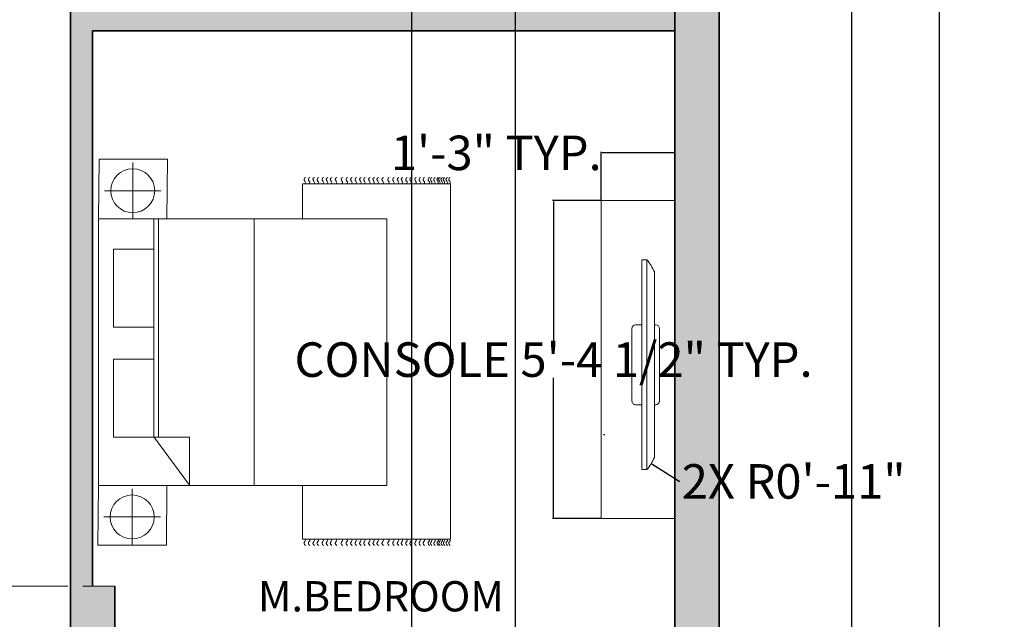
# Model space of a CAD drawing. Units: inches. Extents: x -17 to 892, y -721 to 172.
# Tile 10 of 11: x 655 to 854, y -115 to 7. Entities that reach past the tile are written whole.
import ezdxf

# ---------------------------------------------------------------- set-up
doc = ezdxf.new("R2010")
doc.units = ezdxf.units.IN
doc.header["$MEASUREMENT"] = 0
doc.linetypes.add('ACAD_ISO02W100', pattern=[15, 12, -3])
doc.layers.get('0').update_dxf_attribs({"color": 14})
for name, color, linetype, lineweight in [('A-ANNO-DIMS', 2, 'Continuous', 18), ('A-AREA-IDEN', 7, 'Continuous', 18), ('A-EQPM', 8, 'Continuous', 18), ('A-FLOR-CASE', 252, 'Continuous', 18), ('A-FLOR-OVHD', 252, 'ACAD_ISO02W100', 18), ('A-WALL-PATT', 14, 'Continuous', 13), ('furniture', 252, 'Continuous', 18), ('walls', 252, 'Continuous', 35)]:
    doc.layers.add(name, color=color, linetype=linetype, lineweight=lineweight)
doc.layers.add('A-COLS-PATT', color=254, linetype='Continuous', lineweight=13, true_color=0xd7ebd2)
doc.styles.get("Standard").update_dxf_attribs({"font": 'arial.ttf'})
doc.dimstyles.get("Standard").update_dxf_attribs({"dimtxt": 7, "dimasz": 0.18, "dimexe": 0.18, "dimexo": 0.0625, "dimgap": 0.09, "dimtad": 0, "dimtih": 1, "dimtoh": 1, "dimzin": 0, "dimdsep": 46, "dimlunit": 3, "dimtxsty": 'Standard', "dimcen": 0.09, "dimadec": 0, "dimazin": 0, "dimtfac": 1, "dimtofl": 0, "dimtmove": 0, "dimatfit": 3, "dimfxl": 1, "dimtolj": 1, "dimtzin": 0, "dimarcsym": 0})

# ---------------------------------------------------------------- blocks, each defined once
blk = doc.blocks.new('CARPET')
at = {"layer": 'furniture'}
for p, q in [((-51.53, -98.11), (-51.53, -55.12)), ((-51.53, -55.12), (-41.27, -55.12)), ((36, -55.12), (51.55, -55.12)), ((51.55, -55.12), (51.55, -98.11)), ((51.55, -98.11), (-51.53, -98.11))]:
    blk.add_line(p, q, dxfattribs=at)
for points, knots in [([(-53.37, -55.99), (-53.22, -55.8), (-52.9, -55.41), (-52.34, -55.8), (-51.89, -56.08), (-51.65, -55.91), (-51.53, -55.83)], [0, 0, 0, 0, 0.653278, 1.290138, 1.740457, 2.114451, 2.114451, 2.114451, 2.114451]), ([(-53.37, -57.26), (-53.22, -57.07), (-52.9, -56.67), (-52.34, -57.07), (-51.89, -57.35), (-51.65, -57.17), (-51.53, -57.1)], [0, 0, 0, 0, 0.653278, 1.290138, 1.740457, 2.114451, 2.114451, 2.114451, 2.114451]), ([(53.37, -55.99), (53.22, -55.8), (52.9, -55.41), (52.34, -55.8), (51.89, -56.08), (51.65, -55.91), (51.53, -55.83)], [0, 0, 0, 0, 0.653278, 1.290138, 1.740457, 2.114451, 2.114451, 2.114451, 2.114451]), ([(53.37, -57.26), (53.22, -57.07), (52.9, -56.67), (52.34, -57.07), (51.89, -57.35), (51.65, -57.17), (51.53, -57.1)], [0, 0, 0, 0, 0.653278, 1.290138, 1.740457, 2.114451, 2.114451, 2.114451, 2.114451]), ([(-53.37, -58.59), (-53.22, -58.4), (-52.9, -58.01), (-52.34, -58.4), (-51.89, -58.68), (-51.65, -58.5), (-51.53, -58.43)], [0, 0, 0, 0, 0.653278, 1.290138, 1.740457, 2.114451, 2.114451, 2.114451, 2.114451]), ([(-53.37, -59.78), (-53.22, -59.58), (-52.9, -59.19), (-52.34, -59.58), (-51.89, -59.86), (-51.65, -59.69), (-51.53, -59.61)], [0, 0, 0, 0, 0.653278, 1.290138, 1.740457, 2.114451, 2.114451, 2.114451, 2.114451]), ([(53.37, -58.59), (53.22, -58.4), (52.9, -58.01), (52.34, -58.4), (51.89, -58.68), (51.65, -58.5), (51.53, -58.43)], [0, 0, 0, 0, 0.653278, 1.290138, 1.740457, 2.114451, 2.114451, 2.114451, 2.114451]), ([(53.37, -59.78), (53.22, -59.58), (52.9, -59.19), (52.34, -59.58), (51.89, -59.86), (51.65, -59.69), (51.53, -59.61)], [0, 0, 0, 0, 0.653278, 1.290138, 1.740457, 2.114451, 2.114451, 2.114451, 2.114451]), ([(-53.37, -61.22), (-53.22, -61.02), (-52.9, -60.63), (-52.34, -61.02), (-51.89, -61.3), (-51.65, -61.13), (-51.53, -61.05)], [0, 0, 0, 0, 0.653278, 1.290138, 1.740457, 2.114451, 2.114451, 2.114451, 2.114451]), ([(-53.37, -62.44), (-53.22, -62.25), (-52.9, -61.86), (-52.34, -62.25), (-51.89, -62.53), (-51.65, -62.36), (-51.53, -62.28)], [0, 0, 0, 0, 0.653278, 1.290138, 1.740457, 2.114451, 2.114451, 2.114451, 2.114451]), ([(53.37, -61.22), (53.22, -61.02), (52.9, -60.63), (52.34, -61.02), (51.89, -61.3), (51.65, -61.13), (51.53, -61.05)], [0, 0, 0, 0, 0.653278, 1.290138, 1.740457, 2.114451, 2.114451, 2.114451, 2.114451]), ([(53.37, -62.44), (53.22, -62.25), (52.9, -61.86), (52.34, -62.25), (51.89, -62.53), (51.65, -62.36), (51.53, -62.28)], [0, 0, 0, 0, 0.653278, 1.290138, 1.740457, 2.114451, 2.114451, 2.114451, 2.114451]), ([(-53.37, -63.63), (-53.22, -63.43), (-52.9, -63.04), (-52.34, -63.43), (-51.89, -63.72), (-51.65, -63.54), (-51.53, -63.46)], [0, 0, 0, 0, 0.653278, 1.290138, 1.740457, 2.114451, 2.114451, 2.114451, 2.114451]), ([(-53.37, -65.07), (-53.22, -64.87), (-52.9, -64.48), (-52.34, -64.87), (-51.89, -65.15), (-51.65, -64.98), (-51.53, -64.9)], [0, 0, 0, 0, 0.653278, 1.290138, 1.740457, 2.114451, 2.114451, 2.114451, 2.114451]), ([(53.37, -63.63), (53.22, -63.43), (52.9, -63.04), (52.34, -63.43), (51.89, -63.72), (51.65, -63.54), (51.53, -63.46)], [0, 0, 0, 0, 0.653278, 1.290138, 1.740457, 2.114451, 2.114451, 2.114451, 2.114451]), ([(53.37, -65.07), (53.22, -64.87), (52.9, -64.48), (52.34, -64.87), (51.89, -65.15), (51.65, -64.98), (51.53, -64.9)], [0, 0, 0, 0, 0.653278, 1.290138, 1.740457, 2.114451, 2.114451, 2.114451, 2.114451]), ([(-53.37, -66.76), (-53.22, -66.56), (-52.9, -66.17), (-52.34, -66.56), (-51.89, -66.84), (-51.65, -66.67), (-51.53, -66.59)], [0, 0, 0, 0, 0.653278, 1.290138, 1.740457, 2.114451, 2.114451, 2.114451, 2.114451]), ([(-53.37, -68.2), (-53.22, -68), (-52.9, -67.61), (-52.34, -68), (-51.89, -68.28), (-51.65, -68.11), (-51.53, -68.03)], [0, 0, 0, 0, 0.653278, 1.290138, 1.740457, 2.114451, 2.114451, 2.114451, 2.114451]), ([(53.37, -66.76), (53.22, -66.56), (52.9, -66.17), (52.34, -66.56), (51.89, -66.84), (51.65, -66.67), (51.53, -66.59)], [0, 0, 0, 0, 0.653278, 1.290138, 1.740457, 2.114451, 2.114451, 2.114451, 2.114451]), ([(53.37, -68.2), (53.22, -68), (52.9, -67.61), (52.34, -68), (51.89, -68.28), (51.65, -68.11), (51.53, -68.03)], [0, 0, 0, 0, 0.653278, 1.290138, 1.740457, 2.114451, 2.114451, 2.114451, 2.114451]), ([(-53.37, -69.53), (-53.22, -69.33), (-52.9, -68.94), (-52.34, -69.33), (-51.89, -69.61), (-51.65, -69.44), (-51.53, -69.36)], [0, 0, 0, 0, 0.653278, 1.290138, 1.740457, 2.114451, 2.114451, 2.114451, 2.114451]), ([(-53.37, -70.79), (-53.22, -70.6), (-52.9, -70.21), (-52.34, -70.6), (-51.89, -70.88), (-51.65, -70.7), (-51.53, -70.63)], [0, 0, 0, 0, 0.653278, 1.290138, 1.740457, 2.114451, 2.114451, 2.114451, 2.114451]), ([(53.37, -69.53), (53.22, -69.33), (52.9, -68.94), (52.34, -69.33), (51.89, -69.61), (51.65, -69.44), (51.53, -69.36)], [0, 0, 0, 0, 0.653278, 1.290138, 1.740457, 2.114451, 2.114451, 2.114451, 2.114451]), ([(53.37, -70.79), (53.22, -70.6), (52.9, -70.21), (52.34, -70.6), (51.89, -70.88), (51.65, -70.7), (51.53, -70.63)], [0, 0, 0, 0, 0.653278, 1.290138, 1.740457, 2.114451, 2.114451, 2.114451, 2.114451]), ([(-53.37, -72.12), (-53.22, -71.93), (-52.9, -71.54), (-52.34, -71.93), (-51.89, -72.21), (-51.65, -72.04), (-51.53, -71.96)], [0, 0, 0, 0, 0.653278, 1.290138, 1.740457, 2.114451, 2.114451, 2.114451, 2.114451]), ([(-53.37, -73.31), (-53.22, -73.11), (-52.9, -72.72), (-52.34, -73.11), (-51.89, -73.4), (-51.65, -73.22), (-51.53, -73.14)], [0, 0, 0, 0, 0.653278, 1.290138, 1.740457, 2.114451, 2.114451, 2.114451, 2.114451]), ([(53.37, -72.12), (53.22, -71.93), (52.9, -71.54), (52.34, -71.93), (51.89, -72.21), (51.65, -72.04), (51.53, -71.96)], [0, 0, 0, 0, 0.653278, 1.290138, 1.740457, 2.114451, 2.114451, 2.114451, 2.114451]), ([(53.37, -73.31), (53.22, -73.11), (52.9, -72.72), (52.34, -73.11), (51.89, -73.4), (51.65, -73.22), (51.53, -73.14)], [0, 0, 0, 0, 0.653278, 1.290138, 1.740457, 2.114451, 2.114451, 2.114451, 2.114451]), ([(-53.37, -74.75), (-53.22, -74.55), (-52.9, -74.16), (-52.34, -74.55), (-51.89, -74.83), (-51.65, -74.66), (-51.53, -74.58)], [0, 0, 0, 0, 0.653278, 1.290138, 1.740457, 2.114451, 2.114451, 2.114451, 2.114451]), ([(-53.37, -75.98), (-53.22, -75.78), (-52.9, -75.39), (-52.34, -75.78), (-51.89, -76.06), (-51.65, -75.89), (-51.53, -75.81)], [0, 0, 0, 0, 0.653278, 1.290138, 1.740457, 2.114451, 2.114451, 2.114451, 2.114451]), ([(-53.37, -77.16), (-53.22, -76.96), (-52.9, -76.57), (-52.34, -76.96), (-51.89, -77.25), (-51.65, -77.07), (-51.53, -76.99)], [0, 0, 0, 0, 0.653278, 1.290138, 1.740457, 2.114451, 2.114451, 2.114451, 2.114451]), ([(53.37, -74.75), (53.22, -74.55), (52.9, -74.16), (52.34, -74.55), (51.89, -74.83), (51.65, -74.66), (51.53, -74.58)], [0, 0, 0, 0, 0.653278, 1.290138, 1.740457, 2.114451, 2.114451, 2.114451, 2.114451]), ([(53.37, -75.98), (53.22, -75.78), (52.9, -75.39), (52.34, -75.78), (51.89, -76.06), (51.65, -75.89), (51.53, -75.81)], [0, 0, 0, 0, 0.653278, 1.290138, 1.740457, 2.114451, 2.114451, 2.114451, 2.114451]), ([(53.37, -77.16), (53.22, -76.96), (52.9, -76.57), (52.34, -76.96), (51.89, -77.25), (51.65, -77.07), (51.53, -76.99)], [0, 0, 0, 0, 0.653278, 1.290138, 1.740457, 2.114451, 2.114451, 2.114451, 2.114451]), ([(-53.37, -78.6), (-53.22, -78.4), (-52.9, -78.01), (-52.34, -78.4), (-51.89, -78.68), (-51.65, -78.51), (-51.53, -78.43)], [0, 0, 0, 0, 0.653278, 1.290138, 1.740457, 2.114451, 2.114451, 2.114451, 2.114451]), ([(-53.37, -80.29), (-53.22, -80.09), (-52.9, -79.7), (-52.34, -80.09), (-51.89, -80.37), (-51.65, -80.2), (-51.53, -80.12)], [0, 0, 0, 0, 0.653278, 1.290138, 1.740457, 2.114451, 2.114451, 2.114451, 2.114451]), ([(53.37, -78.6), (53.22, -78.4), (52.9, -78.01), (52.34, -78.4), (51.89, -78.68), (51.65, -78.51), (51.53, -78.43)], [0, 0, 0, 0, 0.653278, 1.290138, 1.740457, 2.114451, 2.114451, 2.114451, 2.114451]), ([(53.37, -80.29), (53.22, -80.09), (52.9, -79.7), (52.34, -80.09), (51.89, -80.37), (51.65, -80.2), (51.53, -80.12)], [0, 0, 0, 0, 0.653278, 1.290138, 1.740457, 2.114451, 2.114451, 2.114451, 2.114451]), ([(-53.37, -81.73), (-53.22, -81.53), (-52.9, -81.14), (-52.34, -81.53), (-51.89, -81.81), (-51.65, -81.64), (-51.53, -81.56)], [0, 0, 0, 0, 0.653278, 1.290138, 1.740457, 2.114451, 2.114451, 2.114451, 2.114451]), ([(-53.37, -83.06), (-53.22, -82.86), (-52.9, -82.47), (-52.34, -82.86), (-51.89, -83.14), (-51.65, -82.97), (-51.53, -82.89)], [0, 0, 0, 0, 0.653278, 1.290138, 1.740457, 2.114451, 2.114451, 2.114451, 2.114451]), ([(53.37, -81.73), (53.22, -81.53), (52.9, -81.14), (52.34, -81.53), (51.89, -81.81), (51.65, -81.64), (51.53, -81.56)], [0, 0, 0, 0, 0.653278, 1.290138, 1.740457, 2.114451, 2.114451, 2.114451, 2.114451]), ([(53.37, -83.06), (53.22, -82.86), (52.9, -82.47), (52.34, -82.86), (51.89, -83.14), (51.65, -82.97), (51.53, -82.89)], [0, 0, 0, 0, 0.653278, 1.290138, 1.740457, 2.114451, 2.114451, 2.114451, 2.114451]), ([(-53.37, -84.18), (-53.22, -83.99), (-52.9, -83.6), (-52.34, -83.99), (-51.89, -84.27), (-51.65, -84.09), (-51.53, -84.02)], [0, 0, 0, 0, 0.653278, 1.290138, 1.740457, 2.114451, 2.114451, 2.114451, 2.114451]), ([(-53.37, -85.51), (-53.22, -85.32), (-52.9, -84.93), (-52.34, -85.32), (-51.89, -85.6), (-51.65, -85.42), (-51.53, -85.35)], [0, 0, 0, 0, 0.653278, 1.290138, 1.740457, 2.114451, 2.114451, 2.114451, 2.114451]), ([(53.37, -84.18), (53.22, -83.99), (52.9, -83.6), (52.34, -83.99), (51.89, -84.27), (51.65, -84.09), (51.53, -84.02)], [0, 0, 0, 0, 0.653278, 1.290138, 1.740457, 2.114451, 2.114451, 2.114451, 2.114451]), ([(53.37, -85.51), (53.22, -85.32), (52.9, -84.93), (52.34, -85.32), (51.89, -85.6), (51.65, -85.42), (51.53, -85.35)], [0, 0, 0, 0, 0.653278, 1.290138, 1.740457, 2.114451, 2.114451, 2.114451, 2.114451]), ([(-53.37, -86.7), (-53.22, -86.5), (-52.9, -86.11), (-52.34, -86.5), (-51.89, -86.78), (-51.65, -86.61), (-51.53, -86.53)], [0, 0, 0, 0, 0.653278, 1.290138, 1.740457, 2.114451, 2.114451, 2.114451, 2.114451]), ([(-53.37, -88.14), (-53.22, -87.94), (-52.9, -87.55), (-52.34, -87.94), (-51.89, -88.22), (-51.65, -88.05), (-51.53, -87.97)], [0, 0, 0, 0, 0.653278, 1.290138, 1.740457, 2.114451, 2.114451, 2.114451, 2.114451]), ([(53.37, -86.7), (53.22, -86.5), (52.9, -86.11), (52.34, -86.5), (51.89, -86.78), (51.65, -86.61), (51.53, -86.53)], [0, 0, 0, 0, 0.653278, 1.290138, 1.740457, 2.114451, 2.114451, 2.114451, 2.114451]), ([(53.37, -88.14), (53.22, -87.94), (52.9, -87.55), (52.34, -87.94), (51.89, -88.22), (51.65, -88.05), (51.53, -87.97)], [0, 0, 0, 0, 0.653278, 1.290138, 1.740457, 2.114451, 2.114451, 2.114451, 2.114451]), ([(-53.37, -89.36), (-53.22, -89.17), (-52.9, -88.78), (-52.34, -89.17), (-51.89, -89.45), (-51.65, -89.28), (-51.53, -89.2)], [0, 0, 0, 0, 0.653278, 1.290138, 1.740457, 2.114451, 2.114451, 2.114451, 2.114451]), ([(-53.37, -90.55), (-53.22, -90.35), (-52.9, -89.96), (-52.34, -90.35), (-51.89, -90.64), (-51.65, -90.46), (-51.53, -90.38)], [0, 0, 0, 0, 0.653278, 1.290138, 1.740457, 2.114451, 2.114451, 2.114451, 2.114451]), ([(53.37, -89.36), (53.22, -89.17), (52.9, -88.78), (52.34, -89.17), (51.89, -89.45), (51.65, -89.28), (51.53, -89.2)], [0, 0, 0, 0, 0.653278, 1.290138, 1.740457, 2.114451, 2.114451, 2.114451, 2.114451]), ([(53.37, -90.55), (53.22, -90.35), (52.9, -89.96), (52.34, -90.35), (51.9, -90.63), (51.66, -90.47), (51.55, -90.4)], [0, 0, 0, 0, 0.653278, 1.290138, 1.740457, 2.0926, 2.0926, 2.0926, 2.0926]), ([(-53.37, -91.99), (-53.22, -91.79), (-52.9, -91.4), (-52.34, -91.79), (-51.89, -92.07), (-51.65, -91.9), (-51.53, -91.82)], [0, 0, 0, 0, 0.653278, 1.290138, 1.740457, 2.114451, 2.114451, 2.114451, 2.114451]), ([(-53.37, -92.69), (-53.22, -92.48), (-52.9, -92.08), (-52.35, -92.49), (-51.89, -92.77), (-51.65, -92.6), (-51.53, -92.52)], [0, 0, 0, 0, 0.663904, 1.307406, 1.757725, 2.131719, 2.131719, 2.131719, 2.131719]), ([(-53.37, -93.61), (-53.22, -93.42), (-52.9, -93.03), (-52.34, -93.42), (-51.89, -93.7), (-51.65, -93.52), (-51.53, -93.45)], [0, 0, 0, 0, 0.653278, 1.290138, 1.740457, 2.114451, 2.114451, 2.114451, 2.114451]), ([(-53.37, -94.55), (-53.22, -94.35), (-52.9, -93.96), (-52.34, -94.35), (-51.89, -94.63), (-51.65, -94.46), (-51.53, -94.38)], [0, 0, 0, 0, 0.653278, 1.290138, 1.740457, 2.114451, 2.114451, 2.114451, 2.114451]), ([(53.37, -91.99), (53.22, -91.79), (52.9, -91.4), (52.34, -91.79), (51.9, -92.07), (51.66, -91.91), (51.55, -91.83)], [0, 0, 0, 0, 0.653278, 1.290138, 1.740457, 2.0926, 2.0926, 2.0926, 2.0926]), ([(53.37, -92.69), (53.22, -92.49), (52.9, -92.09), (52.34, -92.49), (51.9, -92.77), (51.66, -92.61), (51.55, -92.53)], [0, 0, 0, 0, 0.656792, 1.295826, 1.746145, 2.098292, 2.098292, 2.098292, 2.098292]), ([(53.37, -93.66), (53.22, -93.46), (52.9, -93.07), (52.34, -93.46), (51.9, -93.74), (51.66, -93.58), (51.55, -93.5)], [0, 0, 0, 0, 0.653278, 1.290138, 1.740457, 2.0926, 2.0926, 2.0926, 2.0926]), ([(53.37, -94.59), (53.22, -94.4), (52.9, -94.01), (52.34, -94.4), (51.9, -94.68), (51.66, -94.51), (51.55, -94.44)], [0, 0, 0, 0, 0.653278, 1.290138, 1.740457, 2.0926, 2.0926, 2.0926, 2.0926]), ([(-53.37, -95.05), (-53.22, -94.85), (-52.9, -94.46), (-52.34, -94.85), (-51.89, -95.14), (-51.65, -94.96), (-51.53, -94.88)], [0, 0, 0, 0, 0.653278, 1.290138, 1.740457, 2.114451, 2.114451, 2.114451, 2.114451]), ([(-53.37, -95.73), (-53.22, -95.54), (-52.9, -95.15), (-52.34, -95.54), (-51.89, -95.82), (-51.65, -95.65), (-51.53, -95.57)], [0, 0, 0, 0, 0.653278, 1.290138, 1.740457, 2.114451, 2.114451, 2.114451, 2.114451]), ([(-53.37, -96.38), (-53.22, -96.18), (-52.9, -95.79), (-52.34, -96.18), (-51.89, -96.47), (-51.65, -96.29), (-51.53, -96.21)], [0, 0, 0, 0, 0.653278, 1.290138, 1.740457, 2.114451, 2.114451, 2.114451, 2.114451]), ([(-53.37, -97.17), (-53.22, -96.98), (-52.9, -96.59), (-52.34, -96.98), (-51.89, -97.26), (-51.65, -97.08), (-51.53, -97.01)], [0, 0, 0, 0, 0.653278, 1.290138, 1.740457, 2.114451, 2.114451, 2.114451, 2.114451]), ([(53.37, -95.78), (53.22, -95.58), (52.9, -95.19), (52.34, -95.58), (51.89, -95.86), (51.65, -95.69), (51.53, -95.61)], [0, 0, 0, 0, 0.653278, 1.290138, 1.740457, 2.114451, 2.114451, 2.114451, 2.114451]), ([(53.37, -96.43), (53.22, -96.23), (52.9, -95.84), (52.34, -96.23), (51.89, -96.51), (51.65, -96.34), (51.53, -96.26)], [0, 0, 0, 0, 0.653278, 1.290138, 1.740457, 2.114451, 2.114451, 2.114451, 2.114451]), ([(53.37, -97.22), (53.22, -97.02), (52.9, -96.63), (52.34, -97.02), (51.89, -97.3), (51.65, -97.13), (51.53, -97.05)], [0, 0, 0, 0, 0.653278, 1.290138, 1.740457, 2.114451, 2.114451, 2.114451, 2.114451]), ([(53.37, -95.1), (53.22, -94.9), (52.9, -94.51), (52.34, -94.9), (51.9, -95.18), (51.66, -95.02), (51.55, -94.94)], [0, 0, 0, 0, 0.653278, 1.290138, 1.740457, 2.0926, 2.0926, 2.0926, 2.0926]), ([(-53.37, -97.99), (-53.22, -97.79), (-52.9, -97.4), (-52.34, -97.79), (-51.89, -98.08), (-51.65, -97.9), (-51.53, -97.82)], [0, 0, 0, 0, 0.653278, 1.290138, 1.740457, 2.114451, 2.114451, 2.114451, 2.114451]), ([(53.37, -97.99), (53.22, -97.79), (52.9, -97.4), (52.34, -97.79), (51.89, -98.08), (51.65, -97.9), (51.53, -97.82)], [0, 0, 0, 0, 0.653278, 1.290138, 1.740457, 2.114451, 2.114451, 2.114451, 2.114451])]:
    blk.add_open_spline(points, degree=3, knots=knots, dxfattribs=at)
blk = doc.blocks.new('A$C58D270C6')
at = {"layer": 'furniture'}
for p, q in [((9.09, 124.13), (9.09, 108.87)), ((1.46, 116.5), (16.73, 116.5)), ((14.97, 94.84), (24.62, 107.92)), ((24.62, 94.93), (24.62, 107.92)), ((42.08, 108), (42.08, 36)), ((14.97, 94.93), (24.62, 94.93)), ((14.97, 94.84), (14.97, 36)), ((16.22, 94.93), (16.22, 36)), ((9.25, 36), (9.25, 20.74)), ((1.62, 28.37), (16.88, 28.37))]:
    blk.add_line(p, q, dxfattribs=at)
for points in [[(18.5, 108), (18.34, 124.13), (-0.16, 124.13), (0, 108)], [(0, 108), (77.91, 108), (77.91, 36), (0, 36)], [(4.09, 94.93), (14.97, 94.93), (14.97, 73.83), (4.09, 73.83)], [(4.09, 65.23), (14.97, 65.23), (14.97, 44.13), (4.09, 44.13)], [(18.65, 19.87), (18.5, 36), (0, 36), (0.16, 19.87)]]:
    blk.add_lwpolyline(points, close=True, dxfattribs=at)
for centre in [(9.09, 116.5), (9.25, 28.37)]:
    blk.add_circle(centre, 5.95, dxfattribs=at)
at = {"layer": 'furniture', "xscale": 0.9312884925094044, "yscale": 0.9312884925094044, "zscale": 0.9312884925094044, "rotation": 90}
blk.add_blockref('CARPET', (3.79, 74.47), dxfattribs=at)
blk = doc.blocks.new('PLASMA-LARGE')
at = {"layer": 'furniture'}
for p, q in [((-7.26, 0), (7.26, 0)), ((-18.61, -1), (18.61, -1)), ((-8, -1), (-8, -0.74)), ((8, -1), (8, -0.74)), ((-21, -2.5), (21, -2.5)), ((-21, -2.5), (-21, -3.5)), ((-21, -3.5), (21, -3.5)), ((-8, -3.5), (-8, -4.76)), ((8, -3.5), (8, -4.76)), ((21, -2.5), (21, -3.5)), ((-7.26, -5.5), (7.26, -5.5))]:
    blk.add_line(p, q, dxfattribs=at)
for centre, radius, start, end in [((-7.26, -0.74), 0.744, 90, 180), ((7.26, -0.74), 0.744, 0, 90), ((-13.97, -11.05), 11.07, 114.7602, 129.4175), ((13.97, -11.05), 11.07, 50.5825, 65.2398), ((-7.26, -4.76), 0.744, 180, 270), ((7.26, -4.76), 0.744, 270, 0)]:
    blk.add_arc(centre, radius, start, end, dxfattribs=at)
blk = doc.blocks.new('*D17')
at = {"layer": 'A-ANNO-DIMS', "color": 0, "lineweight": -2, "transparency": 16777216}
for p, q in [((822.86, 89.9), (823.61, 89.9)), ((823.43, 89.72), (823.43, -263.08)), ((823.43, -623.21), (823.43, -270.41)), ((822.86, -623.39), (823.61, -623.39))]:
    blk.add_line(p, q, dxfattribs=at)
at = {"layer": 'A-ANNO-DIMS', "color": 0, "lineweight": 100, "transparency": 16777216}
for points in [[(823.4, 89.72), (823.46, 89.72), (823.43, 89.9)], [(823.4, -623.21), (823.46, -623.21), (823.43, -623.39)]]:
    blk.add_solid(points, dxfattribs=at)
at = {"layer": 'Defpoints', "color": 0, "lineweight": 100, "transparency": 16777216}
for p in [(822.8, 89.9), (822.8, -623.39), (823.43, -623.39)]:
    blk.add_point(p, dxfattribs=at)
at = {"layer": 'A-ANNO-DIMS', "color": 0, "transparency": 16777216, "insert": (823.43, -266.74), "char_height": 7, "attachment_point": 5}
blk.add_mtext('\\A1;57\'-1"', dxfattribs=at)
blk = doc.blocks.new('MEDIA-CONSOLE')
for p, q in [((14.9, 64.44), (0, 64.44)), ((14.9, 0), (14.9, 64.44)), ((0, 0), (14.9, 0))]:
    blk.add_line(p, q)
blk = doc.blocks.new('*D36')
at = {"layer": 'A-ANNO-DIMS', "color": 0, "lineweight": -2, "transparency": 16777216}
for p, q in [((772.62, -29.79), (762.83, -29.79)), ((763.01, -29.97), (763.01, -58.3)), ((763.01, -94.05), (763.01, -65.72)), ((772.62, -94.23), (762.83, -94.23))]:
    blk.add_line(p, q, dxfattribs=at)
at = {"layer": 'A-ANNO-DIMS', "color": 0, "lineweight": 100, "transparency": 16777216}
for points in [[(762.98, -29.97), (763.04, -29.97), (763.01, -29.79)], [(762.98, -94.05), (763.04, -94.05), (763.01, -94.23)]]:
    blk.add_solid(points, dxfattribs=at)
at = {"layer": 'Defpoints', "color": 0, "lineweight": 100, "transparency": 16777216}
for p in [(772.68, -29.79), (763.01, -94.23), (772.68, -94.23)]:
    blk.add_point(p, dxfattribs=at)
at = {"layer": 'A-ANNO-DIMS', "color": 0, "transparency": 16777216, "insert": (763.01, -62.01), "char_height": 7, "attachment_point": 5}
blk.add_mtext('\\A1;CONSOLE 5\'-4 1/2" TYP.', dxfattribs=at)
blk = doc.blocks.new('*D37')
at = {"layer": 'A-ANNO-DIMS', "color": 0, "lineweight": -2, "transparency": 16777216}
for p, q in [((772.68, -29.72), (772.68, -19.94)), ((787.58, -29.72), (787.58, -19.94)), ((772.68, -20.12), (772.5, -20.12)), ((787.4, -20.12), (772.86, -20.12))]:
    blk.add_line(p, q, dxfattribs=at)
at = {"layer": 'A-ANNO-DIMS', "color": 0, "lineweight": 100, "transparency": 16777216}
for points in [[(772.86, -20.09), (772.86, -20.15), (772.68, -20.12)], [(787.4, -20.09), (787.4, -20.15), (787.58, -20.12)]]:
    blk.add_solid(points, dxfattribs=at)
at = {"layer": 'Defpoints', "color": 0, "lineweight": 100, "transparency": 16777216}
for p in [(772.68, -20.12), (772.68, -29.79), (787.58, -29.79)]:
    blk.add_point(p, dxfattribs=at)
at = {"layer": 'A-ANNO-DIMS', "color": 0, "transparency": 16777216, "insert": (751.4, -20.12), "char_height": 7, "attachment_point": 5}
blk.add_mtext('\\A1;1\'-3" TYP.', dxfattribs=at)
blk = doc.blocks.new('*D59')
at = {"layer": 'A-ANNO-DIMS', "color": 0, "lineweight": -2, "transparency": 16777216}
for p, q in [((796.64, 89.9), (841.36, 89.9)), ((841.18, 89.72), (841.18, -281.05)), ((841.18, -659.16), (841.18, -288.38)), ((796.64, -659.34), (841.36, -659.34))]:
    blk.add_line(p, q, dxfattribs=at)
at = {"layer": 'A-ANNO-DIMS', "color": 0, "lineweight": 100, "transparency": 16777216}
for points in [[(841.15, 89.72), (841.21, 89.72), (841.18, 89.9)], [(841.15, -659.16), (841.21, -659.16), (841.18, -659.34)]]:
    blk.add_solid(points, dxfattribs=at)
at = {"layer": 'Defpoints', "color": 0, "lineweight": 100, "transparency": 16777216}
for p in [(796.58, 89.9), (841.18, 89.9), (796.58, -659.34)]:
    blk.add_point(p, dxfattribs=at)
at = {"layer": 'A-ANNO-DIMS', "color": 0, "transparency": 16777216, "insert": (841.18, -284.72), "char_height": 7, "attachment_point": 5}
blk.add_mtext('\\A1;62\'-5"', dxfattribs=at)
blk = doc.blocks.new('*D67')
at = {"layer": 'A-ANNO-DIMS', "color": 0, "lineweight": -2, "transparency": 16777216}
for p, q in [((734.21, 32.4), (734.21, -704.12)), ((755.21, 32.4), (755.21, -704.12)), ((734.39, -703.94), (735.64, -703.94)), ((755.03, -703.94), (753.77, -703.94))]:
    blk.add_line(p, q, dxfattribs=at)
at = {"layer": 'A-ANNO-DIMS', "color": 0, "lineweight": 100, "transparency": 16777216}
for points in [[(734.39, -703.91), (734.39, -703.97), (734.21, -703.94)], [(755.03, -703.91), (755.03, -703.97), (755.21, -703.94)]]:
    blk.add_solid(points, dxfattribs=at)
at = {"layer": 'Defpoints', "color": 0, "lineweight": 100, "transparency": 16777216}
for p in [(734.21, 32.46), (755.21, 32.46), (755.21, -703.94)]:
    blk.add_point(p, dxfattribs=at)
at = {"layer": 'A-ANNO-DIMS', "color": 0, "transparency": 16777216, "insert": (744.71, -703.94), "char_height": 7, "attachment_point": 5}
blk.add_mtext('\\A1;1\'-9"', dxfattribs=at)
blk = doc.blocks.new('*D70')
at = {"layer": 'A-ANNO-DIMS', "color": 0, "lineweight": -2, "transparency": 16777216}
for p, q in [((773.2, -77.18), (773.38, -77.18)), ((773.29, -77.27), (773.29, -77.09)), ((788.46, -86.69), (782.92, -83.22)), ((788.64, -86.69), (788.46, -86.69))]:
    blk.add_line(p, q, dxfattribs=at)
at = {"layer": 'A-ANNO-DIMS', "color": 0, "lineweight": 100, "transparency": 16777216}
blk.add_solid([(782.94, -83.19), (782.91, -83.25), (782.77, -83.12)], dxfattribs=at)
at = {"layer": 'Defpoints', "color": 0, "lineweight": 100, "transparency": 16777216}
for p in [(773.29, -77.18), (782.77, -83.12)]:
    blk.add_point(p, dxfattribs=at)
at = {"layer": 'A-ANNO-DIMS', "color": 0, "transparency": 16777216, "insert": (811.68, -86.69), "char_height": 7, "attachment_point": 5}
blk.add_mtext('\\A1;2X R0\'-11"', dxfattribs=at)

msp = doc.modelspace()

# ---------------------------------------------------------------- hatches: boundary and pattern name
at = {"layer": 'A-COLS-PATT'}
h = msp.add_hatch(color=256, dxfattribs=at)
h.dxf.hatch_style = 1
h.paths.add_polyline_path([(796.576, 61.611), (787.576, 61.611), (787.576, 43.692), (796.576, 43.692)])
h.paths.add_polyline_path([(796.576, -140.181), (787.576, -140.181), (787.576, -157.529), (796.576, -157.529)])
h.paths.add_polyline_path([(674.076, -107.889), (665.076, -107.889), (665.076, -116.615), (674.076, -116.615)])
h.paths.add_polyline_path([(537.076, -107.889), (532.576, -107.889), (532.576, -116.615), (537.076, -116.615)])
h.paths.add_polyline_path([(541.576, -207.597), (532.576, -207.597), (532.576, -223.04), (541.576, -223.04)])
h.paths.add_polyline_path([(541.576, -335.389), (532.576, -335.389), (532.576, -350.421), (541.576, -350.421)])
h.paths.add_polyline_path([(541.576, -412.049), (532.576, -412.049), (532.576, -420.971), (541.576, -420.971)])
h.paths.add_polyline_path([(674.076, -410.999), (665.076, -410.999), (665.076, -421.003), (674.076, -421.003)])
h.paths.add_polyline_path([(674.076, -329.432), (665.076, -329.432), (665.076, -335.389), (665.076, -343.822), (674.076, -343.822), (674.076, -335.389)])
h.paths.add_polyline_path([(667.076, -610.134), (659.076, -610.134), (659.076, -618.889), (659.101, -623.389), (667.076, -623.389)])
h.paths.add_polyline_path([(796.576, -610.134), (787.576, -610.134), (787.576, -614.389), (787.576, -623.342), (796.576, -623.342)])
h.paths.add_polyline_path([(796.576, -324.682), (787.576, -324.682), (787.576, -353.487), (796.576, -353.487)])
at = {"layer": 'A-WALL-PATT'}
h = msp.add_hatch(color=256, dxfattribs=at)
h.dxf.hatch_style = 1
h.paths.add_polyline_path([(669.576, 4.611), (787.576, 4.611), (787.576, 9.111), (669.576, 9.111), (669.576, 53.097), (665.076, 53.097), (665.076, -107.889), (669.576, -107.889)])
h.paths.add_polyline_path([(674.076, -116.615), (665.076, -116.615), (665.076, -154.389), (674.076, -154.389)])
h.paths.add_polyline_path([(787.576, -145.389), (713.344, -145.389), (713.344, -154.389), (787.576, -154.389)])
h.paths.add_polyline_path([(632.137, -145.389), (622.476, -145.389), (622.476, -154.389), (632.137, -154.389)])
h.paths.add_polyline_path([(554.583, -145.389), (537.076, -145.389), (537.076, -154.389), (554.583, -154.389)])
h.paths.add_polyline_path([(537.076, -145.389), (532.576, -145.389), (532.576, -154.389), (537.076, -154.389)])
h.paths.add_polyline_path([(537.076, -116.615), (532.576, -116.615), (532.576, -145.389), (537.076, -145.389)])
h.paths.add_polyline_path([(796.576, 43.692), (787.576, 43.692), (787.576, -140.181), (796.576, -140.181)])
h.paths.add_polyline_path([(541.576, -223.04), (532.576, -223.04), (532.576, -282.182), (537.076, -282.182), (541.576, -282.182)])
h.paths.add_polyline_path([(796.576, -157.529), (787.576, -157.529), (787.576, -324.682), (796.576, -324.682)])
h.paths.add_polyline_path([(554.583, -335.389), (541.576, -335.389), (541.576, -344.389), (554.583, -344.389)])
h.paths.add_polyline_path([(635.731, -335.389), (622.476, -335.389), (622.476, -344.389), (635.731, -344.389)])
h.paths.add_polyline_path([(541.576, -350.421), (532.576, -350.421), (532.576, -412.049), (541.576, -412.049)])
h.paths.add_polyline_path([(674.076, -343.822), (665.076, -343.822), (665.076, -410.999), (674.076, -410.999)])
h.paths.add_polyline_path([(667.076, -421.003), (665.076, -421.003), (659.076, -421.002), (659.076, -610.134), (667.076, -610.134)])
h.paths.add_polyline_path([(796.576, -353.487), (787.576, -353.487), (787.576, -610.134), (796.576, -610.134)])
h.paths.add_polyline_path([(787.576, -335.389), (775.362, -335.389), (775.362, -344.389), (787.576, -344.389)])
h.paths.add_polyline_path([(707.469, -335.389), (703.501, -335.389), (703.501, -344.389), (707.469, -344.389)])
h.paths.add_polyline_path([(695.494, 61.611), (676.541, 61.611), (676.541, 57.111), (695.494, 57.111)])
h.paths.add_polyline_path([(729.183, 61.611), (724.076, 61.611), (711.12, 61.611), (711.12, 57.111), (729.183, 57.111)])
h.paths.add_polyline_path([(787.576, 61.611), (735.904, 61.611), (735.904, 57.111), (787.576, 57.111)])

# ---------------------------------------------------------------- linework, layer by layer
at = {"layer": 'A-FLOR-OVHD'}
msp.add_line((532.576, -107.889), (674.076, -107.889), dxfattribs=at)
at = {"layer": 'walls'}
for p, q in [((787.576, 61.611), (787.576, -614.389)), ((796.576, 61.611), (796.576, -623.389)), ((665.076, -107.889), (665.076, 53.097)), ((669.576, 4.611), (787.576, 4.611)), ((669.576, -107.889), (669.576, 4.611)), ((665.076, -154.389), (665.076, -107.889)), ((674.076, -154.389), (674.076, -107.889))]:
    msp.add_line(p, q, dxfattribs=at)

# ---------------------------------------------------------------- block references
at = {"layer": 'A-EQPM', "xscale": 1.011294184530666, "yscale": 1.011294184530666, "zscale": 1.011294184530666, "rotation": 270}
msp.add_blockref('PLASMA-LARGE', (784.465, -63.047), dxfattribs=at)
at = {"layer": 'A-FLOR-CASE', "rotation": 180}
msp.add_blockref('MEDIA-CONSOLE', (787.576, -29.786), dxfattribs=at)
at = {"layer": 'furniture', "xscale": -0.7500000390647866, "yscale": 0.7500000390647866, "zscale": 0.7500000390647866, "rotation": 180}
msp.add_blockref('A$C58D270C6', (670.774, -6.514), dxfattribs=at)

# ---------------------------------------------------------------- texts
at = {"layer": 'A-AREA-IDEN'}
msp.add_text('M.BEDROOM', height=6.1361, dxfattribs=at).set_placement((703.094, -113.028))

# ---------------------------------------------------------------- dimensions: what is measured, and where the dimension line sits
at = {"layer": 'A-ANNO-DIMS'}
dim = msp.add_linear_dim(base=(841.176, 89.902), p1=(796.576, -659.336), p2=(796.576, 89.902), angle=90, dimstyle='Standard', override={"dimdec": 1, "dimlfac": 1, "dimrnd": 0, "dimzin": 1, "dimdsep": 46, "dimlunit": 4, "dimfrac": 2}, dxfattribs=at)
dim.commit()
dim.dimension.update_dxf_attribs({"geometry": '*D59', "text_midpoint": (841.176, -284.717)})
for base, p1, p2, angle, text, override, picture, middle in [((823.427, -623.389), (822.802, 89.902), (822.802, -623.389), 90, '57\'-1"', {"dimclrd": 0, "dimclre": 0, "dimclrt": 0}, '*D17', (823.427, -266.744)), ((772.679, -20.12), (787.576, -29.786), (772.679, -29.786), 180, '<> TYP.', {"dimdec": 1, "dimlfac": 1, "dimrnd": 0, "dimzin": 1, "dimdsep": 46, "dimlunit": 4, "dimfrac": 2}, '*D37', (751.404, -20.12)), ((763.013, -94.229), (772.679, -29.786), (772.679, -94.229), 270, 'CONSOLE <> TYP.', {"dimdec": 1, "dimlfac": 1, "dimrnd": 0, "dimzin": 1, "dimdsep": 46, "dimlunit": 4, "dimfrac": 2}, '*D36', (763.013, -62.008))]:
    dim = msp.add_linear_dim(base=base, p1=p1, p2=p2, angle=angle, text=text, dimstyle='Standard', override=override, dxfattribs=at)
    dim.commit()
    dim.dimension.update_dxf_attribs({"geometry": picture, "text_midpoint": middle})
dim = msp.add_linear_dim(base=(755.209, -703.936), p1=(734.209, 32.461), p2=(755.209, 32.461), dimstyle='Standard', override={"dimdec": 1, "dimlfac": 1, "dimrnd": 0, "dimzin": 1, "dimdsep": 46, "dimlunit": 4, "dimfrac": 2}, dxfattribs=at)
dim.commit()
dim.dimension.update_dxf_attribs({"geometry": '*D67', "text_midpoint": (744.709, -703.936)})
dim = msp.add_radius_dim(center=(773.289, -77.178), mpoint=(782.772, -83.124), text='2X <>', dimstyle='Standard', override={"dimdec": 1, "dimlfac": 1, "dimrnd": 0, "dimzin": 1, "dimdsep": 46, "dimlunit": 4, "dimfrac": 2}, dxfattribs=at)
dim.commit()
dim.dimension.update_dxf_attribs({"geometry": '*D70', "text_midpoint": (811.684, -86.692), "dimtype": 164})

doc.saveas('drawing.dxf')
